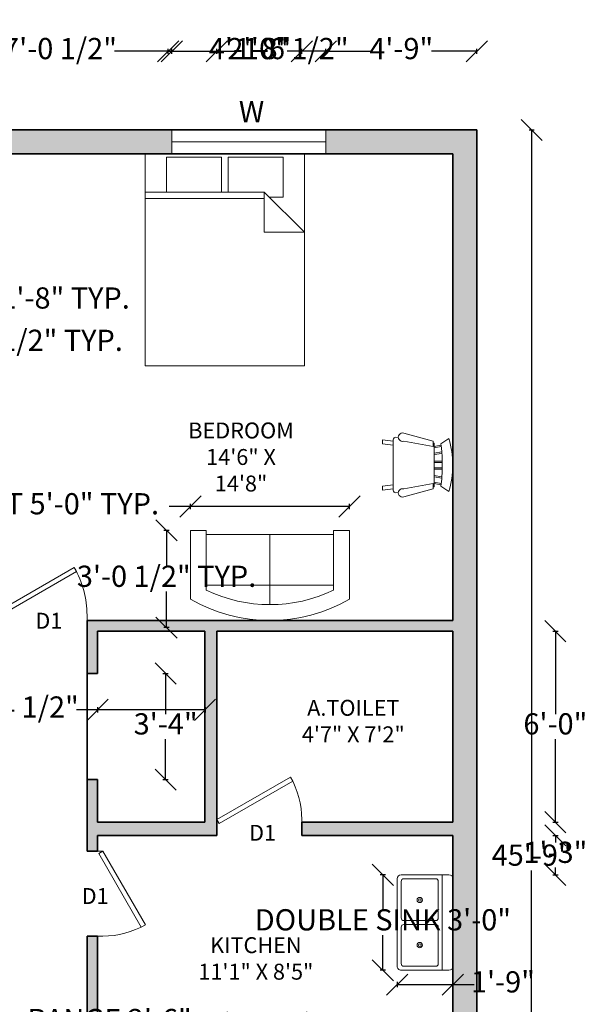
# Model space of a CAD drawing. Units: inches. Extents: x 2530 to 3100, y 543 to 1175.
# Tile 5 of 5: x 2883 to 3097, y 804 to 1175. Entities that reach past the tile are written whole.
import ezdxf

# ---------------------------------------------------------------- set-up
doc = ezdxf.new("R2010")
doc.units = ezdxf.units.IN
for name, color, linetype, lineweight in [('A-ANNO-DIMS', 2, 'Continuous', 18), ('A-ANNO-TEXT', 7, 'Continuous', 18), ('A-AREA-IDEN', 7, 'Continuous', 18), ('A-DOOR', 3, 'Continuous', 18), ('A-FLOR-FIXT', 8, 'Continuous', 18), ('A-FURN', 8, 'Continuous', 18), ('A-GLAZ', 4, 'Continuous', 18), ('A-WALL', 7, 'Continuous', 35), ('A-WALL-PATT', 30, 'Continuous', 13)]:
    doc.layers.add(name, color=color, linetype=linetype, lineweight=lineweight)
doc.styles.get("Standard").update_dxf_attribs({"font": 'arial.ttf'})
doc.dimstyles.new('ISO-25', dxfattribs={"dimtxt": 8, "dimasz": 8, "dimexe": 1, "dimexo": 1, "dimtad": 0, "dimtih": 1, "dimtoh": 1, "dimlunit": 3, "dimtxsty": 'Standard', "dimblk": 'OBLIQUE', "dimcen": 2.5, "dimadec": 0, "dimazin": 0, "dimtfac": 1, "dimtmove": 0, "dimatfit": 3, "dimfxl": 1, "dimfxlon": 1, "dimarcsym": 0})

# ---------------------------------------------------------------- blocks, each defined once
blk = doc.blocks.new('*U7')
for p, q in [((0, 0), (0, -6)), ((32, 0), (32, -6))]:
    blk.add_line(p, q)
blk.add_lwpolyline([(0, 0), (27.71, 16), (28.59, 14.48), (0.87, -1.52)], close=True)
blk.add_arc((0, 0), 32, 0, 30)
blk = doc.blocks.new('*U4')
for p, q in [((0, 0), (0, -6)), ((36, 0), (36, -6))]:
    blk.add_line(p, q)
blk.add_lwpolyline([(0, 0), (31.18, 18), (32.05, 16.48), (0.87, -1.52)], close=True)
blk.add_arc((0, 0), 36, 0, 30)
blk = doc.blocks.new('_Oblique')
at = {"color": 0, "linetype": 'ByBlock', "lineweight": -2}
blk.add_line((-0.5, -0.5), (0.5, 0.5), dxfattribs=at)
blk = doc.blocks.new('*D12')
at = {"layer": 'A-ANNO-DIMS', "color": 0, "lineweight": -2, "transparency": 16777216}
for p, q in [((3074.63, 1133.41), (3076.63, 1133.41)), ((3075.63, 1133.41), (3075.63, 863.62)), ((3075.63, 584.41), (3075.63, 854.2)), ((3074.63, 584.41), (3076.63, 584.41))]:
    blk.add_line(p, q, dxfattribs=at)
at = {"layer": 'Defpoints', "color": 0, "transparency": 16777216}
for p in [(3054.92, 1133.41), (3054.92, 584.41), (3075.63, 584.41)]:
    blk.add_point(p, dxfattribs=at)
at = {"layer": 'A-ANNO-DIMS', "color": 0, "lineweight": -2, "transparency": 16777216, "xscale": 8, "yscale": 8, "zscale": 8}
for p, rotation in [((3075.63, 1133.41), 90), ((3075.63, 584.41), 270)]:
    blk.add_blockref('_Oblique', p, dxfattribs=dict(at, rotation=rotation))
at = {"layer": 'A-ANNO-DIMS', "color": 0, "transparency": 16777216, "insert": (3075.63, 858.91), "char_height": 8, "attachment_point": 5}
blk.add_mtext('45\'-9"', dxfattribs=at)
blk = doc.blocks.new('Sink-double - 36 in top')
for p, q in [((-18, -4), (18, -4)), ((-0.75, -18.5), (-0.75, -6.5)), ((0.75, -6.5), (0.75, -18.5))]:
    blk.add_line(p, q)
for points in [[(-16.5, 0), (16.5, 0)], [(-18, -19.5), (-18, -1.5)], [(18, -1.5), (18, -19.5)], [(-16.5, -18.5), (-16.5, -6.5)], [(-15.5, -5.5), (-1.75, -5.5)], [(1.75, -5.5), (15.5, -5.5)], [(16.5, -6.5), (16.5, -18.5)], [(16.5, -21), (-16.5, -21)], [(-1.75, -19.5), (-15.5, -19.5)], [(15.5, -19.5), (1.75, -19.5)]]:
    blk.add_lwpolyline(points)
for centre, radius in [((-8.5, -12.5), 1), ((-8.5, -12.5), 0.5), ((8.5, -12.5), 1), ((8.5, -12.5), 0.5)]:
    blk.add_circle(centre, radius)
for centre, radius, start, end in [((-16.5, -1.5), 1.5, 90, 180), ((16.5, -1.5), 1.5, 0, 90), ((-15.5, -6.5), 1, 90, 180), ((-1.75, -6.5), 1, 0, 90), ((1.75, -6.5), 1, 90, 180), ((15.5, -6.5), 1, 0, 90), ((-15.5, -18.5), 1, 180, 270), ((-1.75, -18.5), 1, 270, 0), ((1.75, -18.5), 1, 180, 270), ((15.5, -18.5), 1, 270, 0), ((-16.5, -19.5), 1.5, 180, 270), ((16.5, -19.5), 1.5, 270, 0)]:
    blk.add_arc(centre, radius, start, end)
blk = doc.blocks.new('Bed - Queen')
for p, q in [((0, -80.00003), (0, 0)), ((0, 0), (59.99999, 0)), ((59.99999, 0), (59.99999, -80.00003)), ((7.99999, -1.2), (28.79998, -1.2)), ((7.99999, -14.4), (7.99999, -1.2)), ((28.79998, -1.2), (28.79998, -14.4)), ((31.19999, -1.2), (51.99999, -1.2)), ((31.19999, -14.4), (31.19999, -1.2)), ((51.99999, -1.2), (51.99999, -16.4)), ((0, -14.4), (44.8, -14.4)), ((59.99999, -29.6), (44.8, -14.4)), ((44.8, -14.4), (44.8, -29.6)), ((44.8, -16.8), (0, -16.8)), ((51.99999, -16.4), (46.79936, -16.4)), ((44.8, -29.6), (59.99999, -29.6)), ((59.99999, -80.00003), (0, -80.00003))]:
    blk.add_line(p, q)
blk = doc.blocks.new('Sofa - Roundback Loveseat 5 ft.')
for p, q in [((0, -32.44198), (0, -5.99998)), ((-24, -33.99998), (-24, -11.46958)), ((-23.9998, -13.38178), (23.99986, -13.38178)), ((24.00004, -33.99998), (24.00004, -11.46958)), ((-24, -32.44198), (24.00004, -32.44198))]:
    blk.add_line(p, q)
for points in [[(-24, -33.99998), (-30, -33.99998), (-30, -7.99998)], [(30.00004, -7.99998), (30.00004, -33.99998), (24.00004, -33.99998)]]:
    blk.add_lwpolyline(points)
for centre, radius, start, end in [((0, -60.24998), 60.24998, 60.13715, 119.8628), ((0, -61.38438), 55.38444, 64.32083, 115.6792)]:
    blk.add_arc(centre, radius, start, end)
blk = doc.blocks.new('Chair - Rocking')
for p, q in [((-8, -4.5), (-10, -1.5)), ((8, -4.5), (10, -1.5)), ((-8.23428, -6.99939), (-8.3093, -7.47958)), ((-8.23041, -7), (8.23915, -7)), ((-7.5, -4.5), (-7, -7)), ((-6.5, -7), (-7.02225, -4.43)), ((-4.5, -7), (-4.96674, -4.19951)), ((-4, -7), (-4.40532, -4.16272)), ((-1.5, -4.05012), (-1.5, -7)), ((-1, -7), (-1, -4.05012)), ((1, -7), (1, -4.04655)), ((1.5, -4.05012), (1.5, -7)), ((4, -7), (4.40187, -4.18694)), ((4.5, -7), (4.96761, -4.19437)), ((6.5, -7), (7, -4.4057)), ((7.5, -4.5), (7, -7)), ((8.31071, -7.48854), (8.23449, -7.00073)), ((-9, -7.5), (-12, -18.49999)), ((-7, -7.5), (-9, -7.5)), ((-9, -18.49999), (-7, -7.5)), ((7, -7.5), (9, -7.5)), ((9, -18.49999), (7, -7.5)), ((9, -7.5), (12, -18.49999)), ((-10.36644, -20.64523), (-10.5, -21.49999)), ((10.5, -21.49999), (10.3575, -20.58798)), ((-9, -22.49999), (-9.5, -26.49999)), ((0, -22.49999), (-9.5, -22.49999)), ((-8, -26.49999), (-7.5, -22.49999)), ((0, -22.49999), (9.5, -22.49999)), ((8, -26.49999), (7.5, -22.49999)), ((9, -22.49999), (9.5, -26.49999)), ((-9.5, -26.49999), (-8, -26.49999)), ((9.5, -26.49999), (8, -26.49999))]:
    blk.add_line(p, q)
for centre, radius, start, end in [((0, -34.08333), 34.08333, 72.93847, 107.0615), ((0, -68.25004), 64.25, 93.92211, 97.15267), ((0, -68.25004), 64.25, 82.84733, 93.92211), ((-10.5, -18.99999), 1.58114, 161.5651, 18.43495), ((10.5, -18.99999), 1.58114, 161.5651, 18.43495), ((-9.5, -21.49999), 1, 180, 270), ((9.5, -21.49999), 1, 270, 0)]:
    blk.add_arc(centre, radius, start, end)
blk = doc.blocks.new('*D24')
at = {"layer": 'A-ANNO-DIMS', "color": 0, "lineweight": -2, "transparency": 16777216}
for p, q in [((2946.92, 991.41), (2938.92, 991.41)), ((2946.92, 990.41), (2946.92, 992.41)), ((3006.92, 991.41), (2946.92, 991.41)), ((3006.92, 990.41), (3006.92, 992.41))]:
    blk.add_line(p, q, dxfattribs=at)
at = {"layer": 'Defpoints', "color": 0, "transparency": 16777216}
for p in [(2946.92, 991.41), (2946.92, 982.41), (3006.92, 982.41)]:
    blk.add_point(p, dxfattribs=at)
at = {"layer": 'A-ANNO-DIMS', "color": 0, "lineweight": -2, "transparency": 16777216, "xscale": 8, "yscale": 8, "zscale": 8, "rotation": 180}
blk.add_blockref('_Oblique', (2946.92, 991.41), dxfattribs=at)
at = {"layer": 'A-ANNO-DIMS', "color": 0, "lineweight": -2, "transparency": 16777216, "xscale": 8, "yscale": 8, "zscale": 8}
blk.add_blockref('_Oblique', (3006.92, 991.41), dxfattribs=at)
at = {"layer": 'A-ANNO-DIMS', "color": 0, "transparency": 16777216, "insert": (2883.03, 991.41), "char_height": 8, "attachment_point": 5}
blk.add_mtext('LOVESEAT 5\'-0" TYP.', dxfattribs=at)
blk = doc.blocks.new('*D25')
at = {"layer": 'A-ANNO-DIMS', "color": 0, "lineweight": -2, "transparency": 16777216}
for p, q in [((2938.92, 982.41), (2936.92, 982.41)), ((2937.92, 982.41), (2937.92, 968.84)), ((2937.92, 945.74), (2937.92, 959.31)), ((2938.92, 945.74), (2936.92, 945.74))]:
    blk.add_line(p, q, dxfattribs=at)
at = {"layer": 'Defpoints', "color": 0, "transparency": 16777216}
for p in [(2946.92, 982.41), (2937.92, 945.74), (2946.92, 945.74)]:
    blk.add_point(p, dxfattribs=at)
at = {"layer": 'A-ANNO-DIMS', "color": 0, "lineweight": -2, "transparency": 16777216, "xscale": 8, "yscale": 8, "zscale": 8}
for p, rotation in [((2937.92, 982.41), 90), ((2937.92, 945.74), 270)]:
    blk.add_blockref('_Oblique', p, dxfattribs=dict(at, rotation=rotation))
at = {"layer": 'A-ANNO-DIMS', "color": 0, "transparency": 16777216, "insert": (2937.92, 964.07), "char_height": 8, "attachment_point": 5}
blk.add_mtext('3\'-0 1/2" TYP.', dxfattribs=at)
blk = doc.blocks.new('*D30')
at = {"layer": 'A-ANNO-DIMS', "color": 0, "lineweight": -2, "transparency": 16777216}
for p, q in [((2869.69, 1065.33), (2871.69, 1065.33)), ((2870.69, 1065.33), (2870.69, 1057.81)), ((2870.69, 1040.78), (2870.69, 1048.29)), ((2869.69, 1040.78), (2871.69, 1040.78))]:
    blk.add_line(p, q, dxfattribs=at)
at = {"layer": 'Defpoints', "color": 0, "transparency": 16777216}
for p in [(2867.01, 1065.33), (2867.01, 1040.78), (2870.69, 1040.78)]:
    blk.add_point(p, dxfattribs=at)
at = {"layer": 'A-ANNO-DIMS', "color": 0, "lineweight": -2, "transparency": 16777216, "xscale": 8, "yscale": 8, "zscale": 8}
for p, rotation in [((2870.69, 1065.33), 90), ((2870.69, 1040.78), 270)]:
    blk.add_blockref('_Oblique', p, dxfattribs=dict(at, rotation=rotation))
at = {"layer": 'A-ANNO-DIMS', "color": 0, "transparency": 16777216, "insert": (2870.69, 1053.05), "char_height": 8, "attachment_point": 5}
blk.add_mtext('BASIN 2\'-0 1/2" TYP.', dxfattribs=at)
blk = doc.blocks.new('*D31')
at = {"layer": 'A-ANNO-DIMS', "color": 0, "lineweight": -2, "transparency": 16777216}
for p, q in [((2846.87, 1068.01), (2846.87, 1070.01)), ((2867.01, 1068.01), (2867.01, 1070.01)), ((2846.87, 1069.01), (2867.01, 1069.01)), ((2867.01, 1069.01), (2875.01, 1069.01))]:
    blk.add_line(p, q, dxfattribs=at)
at = {"layer": 'Defpoints', "color": 0, "transparency": 16777216}
for p in [(2867.01, 1069.01), (2846.87, 1065.33), (2867.01, 1065.33)]:
    blk.add_point(p, dxfattribs=at)
at = {"layer": 'A-ANNO-DIMS', "color": 0, "lineweight": -2, "transparency": 16777216, "xscale": 8, "yscale": 8, "zscale": 8, "rotation": 180}
blk.add_blockref('_Oblique', (2846.87, 1069.01), dxfattribs=at)
at = {"layer": 'A-ANNO-DIMS', "color": 0, "lineweight": -2, "transparency": 16777216, "xscale": 8, "yscale": 8, "zscale": 8}
blk.add_blockref('_Oblique', (2867.01, 1069.01), dxfattribs=at)
at = {"layer": 'A-ANNO-DIMS', "color": 0, "transparency": 16777216, "insert": (2899.64, 1069.01), "char_height": 8, "attachment_point": 5}
blk.add_mtext('1\'-8" TYP.', dxfattribs=at)
blk = doc.blocks.new('*D34')
at = {"layer": 'A-ANNO-DIMS', "color": 0, "lineweight": -2, "transparency": 16777216}
for p, q in [((3020.52, 852.52), (3018.52, 852.52)), ((3019.52, 852.52), (3019.52, 839.29)), ((3019.52, 816.52), (3019.52, 829.76)), ((3020.52, 816.52), (3018.52, 816.52))]:
    blk.add_line(p, q, dxfattribs=at)
at = {"layer": 'Defpoints', "color": 0, "transparency": 16777216}
for p in [(3024.92, 852.52), (3019.52, 816.52), (3024.92, 816.52)]:
    blk.add_point(p, dxfattribs=at)
at = {"layer": 'A-ANNO-DIMS', "color": 0, "lineweight": -2, "transparency": 16777216, "xscale": 8, "yscale": 8, "zscale": 8}
for p, rotation in [((3019.52, 852.52), 90), ((3019.52, 816.52), 270)]:
    blk.add_blockref('_Oblique', p, dxfattribs=dict(at, rotation=rotation))
at = {"layer": 'A-ANNO-DIMS', "color": 0, "transparency": 16777216, "insert": (3019.52, 834.52), "char_height": 8, "attachment_point": 5}
blk.add_mtext('DOUBLE SINK 3\'-0"', dxfattribs=at)
blk = doc.blocks.new('*D35')
at = {"layer": 'A-ANNO-DIMS', "color": 0, "lineweight": -2, "transparency": 16777216}
for p, q in [((3024.92, 812.12), (3024.92, 810.12)), ((3024.92, 811.12), (3045.92, 811.12)), ((3045.92, 812.12), (3045.92, 810.12)), ((3045.92, 811.12), (3053.92, 811.12))]:
    blk.add_line(p, q, dxfattribs=at)
at = {"layer": 'Defpoints', "color": 0, "transparency": 16777216}
for p in [(3024.92, 816.52), (3045.92, 816.52), (3045.92, 811.12)]:
    blk.add_point(p, dxfattribs=at)
at = {"layer": 'A-ANNO-DIMS', "color": 0, "lineweight": -2, "transparency": 16777216, "xscale": 8, "yscale": 8, "zscale": 8, "rotation": 180}
blk.add_blockref('_Oblique', (3024.92, 811.12), dxfattribs=at)
at = {"layer": 'A-ANNO-DIMS', "color": 0, "lineweight": -2, "transparency": 16777216, "xscale": 8, "yscale": 8, "zscale": 8}
blk.add_blockref('_Oblique', (3045.92, 811.12), dxfattribs=at)
at = {"layer": 'A-ANNO-DIMS', "color": 0, "transparency": 16777216, "insert": (3064.8, 811.12), "char_height": 8, "attachment_point": 5}
blk.add_mtext('1\'-9"', dxfattribs=at)
blk = doc.blocks.new('*D36')
at = {"layer": 'A-ANNO-DIMS', "color": 0, "lineweight": -2, "transparency": 16777216}
for p, q in [((2956.92, 796.91), (2948.92, 796.91)), ((2956.92, 795.91), (2956.92, 797.91)), ((2986.92, 796.91), (2956.92, 796.91)), ((2986.92, 795.91), (2986.92, 797.91))]:
    blk.add_line(p, q, dxfattribs=at)
at = {"layer": 'Defpoints', "color": 0, "transparency": 16777216}
for p in [(2956.92, 796.91), (2956.92, 792.41), (2986.92, 792.41)]:
    blk.add_point(p, dxfattribs=at)
at = {"layer": 'A-ANNO-DIMS', "color": 0, "lineweight": -2, "transparency": 16777216, "xscale": 8, "yscale": 8, "zscale": 8, "rotation": 180}
blk.add_blockref('_Oblique', (2956.92, 796.91), dxfattribs=at)
at = {"layer": 'A-ANNO-DIMS', "color": 0, "lineweight": -2, "transparency": 16777216, "xscale": 8, "yscale": 8, "zscale": 8}
blk.add_blockref('_Oblique', (2986.92, 796.91), dxfattribs=at)
at = {"layer": 'A-ANNO-DIMS', "color": 0, "transparency": 16777216, "insert": (2916.44, 796.91), "char_height": 8, "attachment_point": 5}
blk.add_mtext('RANGE 2\'-6"', dxfattribs=at)
blk = doc.blocks.new('*D38')
at = {"layer": 'A-ANNO-DIMS', "color": 0, "lineweight": -2, "transparency": 16777216}
for p, q in [((2911.92, 791.86), (2903.92, 791.86)), ((2911.92, 790.86), (2911.92, 792.86)), ((2938.56, 791.86), (2911.92, 791.86)), ((2938.56, 790.86), (2938.56, 792.86))]:
    blk.add_line(p, q, dxfattribs=at)
at = {"layer": 'Defpoints', "color": 0, "transparency": 16777216}
for p in [(2911.92, 791.86), (2911.92, 787.87), (2938.56, 787.87)]:
    blk.add_point(p, dxfattribs=at)
at = {"layer": 'A-ANNO-DIMS', "color": 0, "lineweight": -2, "transparency": 16777216, "xscale": 8, "yscale": 8, "zscale": 8, "rotation": 180}
blk.add_blockref('_Oblique', (2911.92, 791.86), dxfattribs=at)
at = {"layer": 'A-ANNO-DIMS', "color": 0, "lineweight": -2, "transparency": 16777216, "xscale": 8, "yscale": 8, "zscale": 8}
blk.add_blockref('_Oblique', (2938.56, 791.86), dxfattribs=at)
at = {"layer": 'A-ANNO-DIMS', "color": 0, "transparency": 16777216, "insert": (2837.6, 791.86), "char_height": 8, "attachment_point": 5}
blk.add_mtext('REFRIGERATOR 2\'-2 1/2"', dxfattribs=at)
blk = doc.blocks.new('*D54')
at = {"layer": 'A-ANNO-DIMS', "color": 0, "lineweight": -2, "transparency": 16777216}
for p, q in [((2855.56, 1162.06), (2855.56, 1164.06)), ((2855.56, 1163.06), (2877.19, 1163.06)), ((2939.91, 1163.06), (2918.28, 1163.06)), ((2939.91, 1162.06), (2939.91, 1164.06))]:
    blk.add_line(p, q, dxfattribs=at)
at = {"layer": 'Defpoints', "color": 0, "transparency": 16777216}
for p in [(2939.91, 1163.06), (2855.56, 1133.41), (2939.91, 1133.41)]:
    blk.add_point(p, dxfattribs=at)
at = {"layer": 'A-ANNO-DIMS', "color": 0, "lineweight": -2, "transparency": 16777216, "xscale": 8, "yscale": 8, "zscale": 8, "rotation": 180}
blk.add_blockref('_Oblique', (2855.56, 1163.06), dxfattribs=at)
at = {"layer": 'A-ANNO-DIMS', "color": 0, "lineweight": -2, "transparency": 16777216, "xscale": 8, "yscale": 8, "zscale": 8}
blk.add_blockref('_Oblique', (2939.91, 1163.06), dxfattribs=at)
at = {"layer": 'A-ANNO-DIMS', "color": 0, "transparency": 16777216, "insert": (2897.74, 1163.06), "char_height": 8, "attachment_point": 5}
blk.add_mtext('7\'-0 1/2"', dxfattribs=at)
blk = doc.blocks.new('*D55')
at = {"layer": 'A-ANNO-DIMS', "color": 0, "lineweight": -2, "transparency": 16777216}
for p, q in [((2939.91, 1162.06), (2939.91, 1164.06)), ((2939.91, 1163.06), (2954.41, 1163.06)), ((2997.97, 1163.06), (2983.47, 1163.06)), ((2997.97, 1162.06), (2997.97, 1164.06))]:
    blk.add_line(p, q, dxfattribs=at)
at = {"layer": 'Defpoints', "color": 0, "transparency": 16777216}
for p in [(2997.97, 1163.06), (2939.91, 1133.41), (2997.97, 1133.41)]:
    blk.add_point(p, dxfattribs=at)
at = {"layer": 'A-ANNO-DIMS', "color": 0, "lineweight": -2, "transparency": 16777216, "xscale": 8, "yscale": 8, "zscale": 8, "rotation": 180}
blk.add_blockref('_Oblique', (2939.91, 1163.06), dxfattribs=at)
at = {"layer": 'A-ANNO-DIMS', "color": 0, "lineweight": -2, "transparency": 16777216, "xscale": 8, "yscale": 8, "zscale": 8}
blk.add_blockref('_Oblique', (2997.97, 1163.06), dxfattribs=at)
at = {"layer": 'A-ANNO-DIMS', "color": 0, "transparency": 16777216, "insert": (2968.94, 1163.06), "char_height": 8, "attachment_point": 5}
blk.add_mtext('4\'-10"', dxfattribs=at)
blk = doc.blocks.new('*D65')
at = {"layer": 'A-ANNO-DIMS', "color": 0, "lineweight": -2, "transparency": 16777216}
for p, q in [((2597.27, 861.41), (2595.27, 861.41)), ((2596.27, 861.41), (2596.27, 850.12)), ((2596.27, 829.41), (2596.27, 840.7)), ((2597.27, 829.41), (2595.27, 829.41))]:
    blk.add_line(p, q, dxfattribs=at)
at = {"layer": 'Defpoints', "color": 0, "transparency": 16777216}
for p in [(2596.27, 861.41), (2907.92, 861.41), (2907.92, 829.41)]:
    blk.add_point(p, dxfattribs=at)
at = {"layer": 'A-ANNO-DIMS', "color": 0, "lineweight": -2, "transparency": 16777216, "xscale": 8, "yscale": 8, "zscale": 8}
for p, rotation in [((2596.27, 861.41), 90), ((2596.27, 829.41), 270)]:
    blk.add_blockref('_Oblique', p, dxfattribs=dict(at, rotation=rotation))
at = {"layer": 'A-ANNO-DIMS', "color": 0, "transparency": 16777216, "insert": (2596.27, 845.41), "char_height": 8, "attachment_point": 5}
blk.add_mtext('2\'-8"', dxfattribs=at)
blk = doc.blocks.new('*D69')
at = {"layer": 'A-ANNO-DIMS', "color": 0, "lineweight": -2, "transparency": 16777216}
for p, q in [((2956.92, 555.76), (2956.92, 553.76)), ((2956.92, 554.76), (2990.19, 554.76)), ((3045.92, 554.76), (3012.64, 554.76)), ((3045.92, 555.76), (3045.92, 553.76))]:
    blk.add_line(p, q, dxfattribs=at)
at = {"layer": 'Defpoints', "color": 0, "transparency": 16777216}
for p in [(2956.92, 944.41), (3045.92, 944.41), (3045.92, 554.76)]:
    blk.add_point(p, dxfattribs=at)
at = {"layer": 'A-ANNO-DIMS', "color": 0, "lineweight": -2, "transparency": 16777216, "xscale": 8, "yscale": 8, "zscale": 8, "rotation": 180}
blk.add_blockref('_Oblique', (2956.92, 554.76), dxfattribs=at)
at = {"layer": 'A-ANNO-DIMS', "color": 0, "lineweight": -2, "transparency": 16777216, "xscale": 8, "yscale": 8, "zscale": 8}
blk.add_blockref('_Oblique', (3045.92, 554.76), dxfattribs=at)
at = {"layer": 'A-ANNO-DIMS', "color": 0, "transparency": 16777216, "insert": (3001.42, 554.76), "char_height": 8, "attachment_point": 5}
blk.add_mtext('7\'-5"', dxfattribs=at)
blk = doc.blocks.new('*D70')
at = {"layer": 'A-ANNO-DIMS', "color": 0, "lineweight": -2, "transparency": 16777216}
for p, q in [((3083.57, 944.41), (3085.57, 944.41)), ((3084.57, 944.41), (3084.57, 913.12)), ((3084.57, 872.41), (3084.57, 903.7)), ((3083.57, 872.41), (3085.57, 872.41))]:
    blk.add_line(p, q, dxfattribs=at)
at = {"layer": 'Defpoints', "color": 0, "transparency": 16777216}
for p in [(3045.92, 944.41), (3084.57, 944.41), (3045.92, 872.41)]:
    blk.add_point(p, dxfattribs=at)
at = {"layer": 'A-ANNO-DIMS', "color": 0, "lineweight": -2, "transparency": 16777216, "xscale": 8, "yscale": 8, "zscale": 8}
for p, rotation in [((3084.57, 944.41), 90), ((3084.57, 872.41), 270)]:
    blk.add_blockref('_Oblique', p, dxfattribs=dict(at, rotation=rotation))
at = {"layer": 'A-ANNO-DIMS', "color": 0, "transparency": 16777216, "insert": (3084.57, 908.41), "char_height": 8, "attachment_point": 5}
blk.add_mtext('6\'-0"', dxfattribs=at)
blk = doc.blocks.new('*D73')
at = {"layer": 'A-ANNO-DIMS', "color": 0, "lineweight": -2, "transparency": 16777216}
for p, q in [((2997.97, 1162.06), (2997.97, 1164.06)), ((2997.97, 1163.06), (3015.02, 1163.06)), ((3054.92, 1163.06), (3037.86, 1163.06)), ((3054.92, 1162.06), (3054.92, 1164.06))]:
    blk.add_line(p, q, dxfattribs=at)
at = {"layer": 'Defpoints', "color": 0, "transparency": 16777216}
for p in [(3054.92, 1163.06), (2997.97, 1133.41), (3054.92, 1133.41)]:
    blk.add_point(p, dxfattribs=at)
at = {"layer": 'A-ANNO-DIMS', "color": 0, "lineweight": -2, "transparency": 16777216, "xscale": 8, "yscale": 8, "zscale": 8, "rotation": 180}
blk.add_blockref('_Oblique', (2997.97, 1163.06), dxfattribs=at)
at = {"layer": 'A-ANNO-DIMS', "color": 0, "lineweight": -2, "transparency": 16777216, "xscale": 8, "yscale": 8, "zscale": 8}
blk.add_blockref('_Oblique', (3054.92, 1163.06), dxfattribs=at)
at = {"layer": 'A-ANNO-DIMS', "color": 0, "transparency": 16777216, "insert": (3026.44, 1163.06), "char_height": 8, "attachment_point": 5}
blk.add_mtext('4\'-9"', dxfattribs=at)
blk = doc.blocks.new('*D75')
at = {"layer": 'A-ANNO-DIMS', "color": 0, "lineweight": -2, "transparency": 16777216}
for p, q in [((2936.57, 928.41), (2938.57, 928.41)), ((2937.57, 928.41), (2937.57, 913.12)), ((2937.57, 888.41), (2937.57, 903.7)), ((2936.57, 888.41), (2938.57, 888.41))]:
    blk.add_line(p, q, dxfattribs=at)
at = {"layer": 'Defpoints', "color": 0, "transparency": 16777216}
for p in [(2907.92, 928.41), (2907.92, 888.41), (2937.57, 888.41)]:
    blk.add_point(p, dxfattribs=at)
at = {"layer": 'A-ANNO-DIMS', "color": 0, "lineweight": -2, "transparency": 16777216, "xscale": 8, "yscale": 8, "zscale": 8}
for p, rotation in [((2937.57, 928.41), 90), ((2937.57, 888.41), 270)]:
    blk.add_blockref('_Oblique', p, dxfattribs=dict(at, rotation=rotation))
at = {"layer": 'A-ANNO-DIMS', "color": 0, "transparency": 16777216, "insert": (2937.57, 908.41), "char_height": 8, "attachment_point": 5}
blk.add_mtext('3\'-4"', dxfattribs=at)
blk = doc.blocks.new('*D76')
at = {"layer": 'A-ANNO-DIMS', "color": 0, "lineweight": -2, "transparency": 16777216}
for p, q in [((2911.92, 914.76), (2903.92, 914.76)), ((2911.92, 915.76), (2911.92, 913.76)), ((2952.42, 914.76), (2911.92, 914.76)), ((2952.42, 915.76), (2952.42, 913.76))]:
    blk.add_line(p, q, dxfattribs=at)
at = {"layer": 'Defpoints', "color": 0, "transparency": 16777216}
for p in [(2911.92, 944.41), (2952.42, 944.41), (2911.92, 914.76)]:
    blk.add_point(p, dxfattribs=at)
at = {"layer": 'A-ANNO-DIMS', "color": 0, "lineweight": -2, "transparency": 16777216, "xscale": 8, "yscale": 8, "zscale": 8}
for p, rotation in [((2911.92, 914.76), 180.000000000001), ((2952.42, 914.76), 1.0392e-12)]:
    blk.add_blockref('_Oblique', p, dxfattribs=dict(at, rotation=rotation))
at = {"layer": 'A-ANNO-DIMS', "color": 0, "transparency": 16777216, "insert": (2883.34, 914.76), "char_height": 8, "attachment_point": 5}
blk.add_mtext('3\'-4 1/2"', dxfattribs=at)
blk = doc.blocks.new('*D77')
at = {"layer": 'A-ANNO-DIMS', "color": 0, "lineweight": -2, "transparency": 16777216}
for p, q in [((2938.56, 1162.06), (2938.56, 1164.06)), ((2938.56, 1163.06), (2956.92, 1163.06)), ((2956.92, 1162.06), (2956.92, 1164.06)), ((2956.92, 1163.06), (2964.92, 1163.06))]:
    blk.add_line(p, q, dxfattribs=at)
at = {"layer": 'Defpoints', "color": 0, "transparency": 16777216}
for p in [(2956.92, 1163.06), (2956.92, 790.41), (2938.56, 787.13)]:
    blk.add_point(p, dxfattribs=at)
at = {"layer": 'A-ANNO-DIMS', "color": 0, "lineweight": -2, "transparency": 16777216, "xscale": 8, "yscale": 8, "zscale": 8, "rotation": 180}
blk.add_blockref('_Oblique', (2938.56, 1163.06), dxfattribs=at)
at = {"layer": 'A-ANNO-DIMS', "color": 0, "lineweight": -2, "transparency": 16777216, "xscale": 8, "yscale": 8, "zscale": 8}
blk.add_blockref('_Oblique', (2956.92, 1163.06), dxfattribs=at)
at = {"layer": 'A-ANNO-DIMS', "color": 0, "transparency": 16777216, "insert": (2985.12, 1163.06), "char_height": 8, "attachment_point": 5}
blk.add_mtext('1\'-6 1/2"', dxfattribs=at)
blk = doc.blocks.new('*D78')
at = {"layer": 'A-ANNO-DIMS', "color": 0, "lineweight": -2, "transparency": 16777216}
for p, q in [((3083.57, 867.41), (3085.57, 867.41)), ((3084.57, 867.41), (3084.57, 864.68)), ((3084.57, 852.52), (3084.57, 855.25)), ((3083.57, 852.52), (3085.57, 852.52))]:
    blk.add_line(p, q, dxfattribs=at)
at = {"layer": 'Defpoints', "color": 0, "transparency": 16777216}
for p in [(3045.92, 867.41), (3084.57, 867.41), (3044.42, 852.52)]:
    blk.add_point(p, dxfattribs=at)
at = {"layer": 'A-ANNO-DIMS', "color": 0, "lineweight": -2, "transparency": 16777216, "xscale": 8, "yscale": 8, "zscale": 8}
for p, rotation in [((3084.57, 867.41), 90), ((3084.57, 852.52), 270)]:
    blk.add_blockref('_Oblique', p, dxfattribs=dict(at, rotation=rotation))
at = {"layer": 'A-ANNO-DIMS', "color": 0, "transparency": 16777216, "insert": (3084.57, 859.97), "char_height": 8, "attachment_point": 5}
blk.add_mtext('1\'-3"', dxfattribs=at)
blk = doc.blocks.new('*D82')
at = {"layer": 'A-ANNO-DIMS', "color": 0, "lineweight": -2, "transparency": 16777216}
for p, q in [((2956.92, 1162.06), (2956.92, 1164.06)), ((2956.92, 1163.06), (2961.59, 1163.06)), ((2988.92, 1163.06), (2984.24, 1163.06)), ((2988.92, 1162.06), (2988.92, 1164.06))]:
    blk.add_line(p, q, dxfattribs=at)
at = {"layer": 'Defpoints', "color": 0, "transparency": 16777216}
for p in [(2988.92, 1163.06), (2956.92, 867.41), (2988.92, 867.41)]:
    blk.add_point(p, dxfattribs=at)
at = {"layer": 'A-ANNO-DIMS', "color": 0, "lineweight": -2, "transparency": 16777216, "xscale": 8, "yscale": 8, "zscale": 8, "rotation": 180}
blk.add_blockref('_Oblique', (2956.92, 1163.06), dxfattribs=at)
at = {"layer": 'A-ANNO-DIMS', "color": 0, "lineweight": -2, "transparency": 16777216, "xscale": 8, "yscale": 8, "zscale": 8}
blk.add_blockref('_Oblique', (2988.92, 1163.06), dxfattribs=at)
at = {"layer": 'A-ANNO-DIMS', "color": 0, "transparency": 16777216, "insert": (2972.92, 1163.06), "char_height": 8, "attachment_point": 5}
blk.add_mtext('2\'-8"', dxfattribs=at)

msp = doc.modelspace()

# ---------------------------------------------------------------- hatches: boundary and pattern name
at = {"layer": 'A-WALL-PATT'}
h = msp.add_hatch(color=256, dxfattribs=at)
h.dxf.hatch_style = 1
h.paths.add_polyline_path([(2676.945, 1133.407), (2625.918, 1133.407), (2625.918, 584.407), (2673.585, 584.407), (2673.585, 593.407), (2634.918, 593.407), (2634.918, 757.407), (2717.918, 757.407), (2717.918, 766.407), (2634.918, 766.407), (2634.918, 944.407), (2772.918, 944.407), (2772.918, 948.407), (2634.918, 948.407), (2634.918, 1124.407), (2676.945, 1124.407)])
h.paths.add_polyline_path([(2822.346, 1133.407), (2739.946, 1133.407), (2739.946, 1124.407), (2808.918, 1124.407), (2808.918, 1070.407), (2812.918, 1070.407), (2812.918, 1124.407), (2822.346, 1124.407)])
h.paths.add_polyline_path([(2939.91, 1133.407), (2855.561, 1133.407), (2855.561, 1124.407), (2867.918, 1124.407), (2867.918, 1038.407), (2808.918, 1038.407), (2808.918, 944.407), (2871.918, 944.407), (2871.918, 1002.407), (2867.918, 1002.407), (2867.918, 948.407), (2812.918, 948.407), (2812.918, 1034.407), (2871.918, 1034.407), (2871.918, 1124.407), (2939.91, 1124.407)])
h.paths.add_polyline_path([(3054.918, 1133.407), (2997.969, 1133.407), (2997.969, 1124.407), (3045.918, 1124.407), (3045.918, 948.407), (2907.918, 948.407), (2907.918, 928.407), (2911.918, 928.407), (2911.918, 944.407), (2952.418, 944.407), (2952.418, 872.407), (2911.918, 872.407), (2911.918, 888.407), (2907.918, 888.407), (2907.918, 861.407), (2911.918, 861.407), (2911.918, 867.407), (2956.918, 867.407), (2956.918, 944.407), (3045.918, 944.407), (3045.918, 872.407), (2988.918, 872.407), (2988.918, 867.407), (3045.918, 867.407), (3045.918, 766.407), (2986.918, 766.407), (2986.918, 757.407), (3045.918, 757.407), (3045.918, 593.407), (2906.263, 593.407), (2906.263, 584.407), (3054.918, 584.407)])
h.paths.add_polyline_path([(2780.418, 593.407), (2762.418, 593.407), (2762.418, 693.907), (2757.918, 693.907), (2757.918, 593.407), (2719.35, 593.407), (2719.35, 584.407), (2780.418, 584.407)])
h.paths.add_polyline_path([(2846.356, 593.407), (2826.918, 593.407), (2826.918, 757.407), (2826.918, 766.407), (2822.418, 766.407), (2822.418, 693.907), (2794.418, 693.907), (2794.418, 689.407), (2822.418, 689.407), (2822.418, 593.407), (2804.418, 593.407), (2804.418, 584.407), (2846.356, 584.407)])
h.paths.add_polyline_path([(2938.918, 766.407), (2911.918, 766.407), (2911.918, 829.407), (2907.918, 829.407), (2907.918, 766.407), (2886.918, 766.407), (2886.918, 757.407), (2938.918, 757.407)])
h.paths.add_polyline_path([(2822.418, 766.407), (2757.918, 766.407), (2757.918, 757.407), (2757.918, 721.407), (2762.418, 721.407), (2762.418, 757.407), (2822.418, 757.407)])

# ---------------------------------------------------------------- linework, layer by layer
at = {"layer": 'A-GLAZ'}
for p, q in [((2939.91, 1124.407), (2939.91, 1133.407)), ((2997.969, 1124.407), (2997.969, 1133.407)), ((2997.969, 1128.907), (2939.91, 1128.907))]:
    msp.add_line(p, q, dxfattribs=at)
at = {"layer": 'A-WALL'}
for p, q in [((3054.918, 1133.407), (2625.918, 1133.407)), ((3054.918, 584.407), (3054.918, 1133.407)), ((3045.918, 1124.407), (2871.918, 1124.407)), ((3045.918, 948.407), (3045.918, 1124.407)), ((3045.918, 948.407), (2907.918, 948.407)), ((2907.918, 861.407), (2907.918, 948.407)), ((2952.418, 944.407), (2911.918, 944.407)), ((2911.918, 928.407), (2911.918, 944.407)), ((2952.418, 872.407), (2952.418, 944.407)), ((3045.918, 944.407), (2956.918, 944.407)), ((2956.918, 867.407), (2956.918, 944.407)), ((3045.918, 872.407), (3045.918, 944.407)), ((2911.918, 928.407), (2907.918, 928.407)), ((2911.918, 888.407), (2907.918, 888.407)), ((2911.918, 872.407), (2911.918, 888.407)), ((2952.418, 872.407), (2911.918, 872.407)), ((3045.918, 872.407), (2988.918, 872.407)), ((2988.918, 867.407), (2988.918, 872.407)), ((2956.918, 867.407), (2911.918, 867.407)), ((2911.918, 861.407), (2911.918, 867.407)), ((3045.918, 867.407), (2988.918, 867.407)), ((3045.918, 766.407), (3045.918, 867.407)), ((2911.918, 861.407), (2907.918, 861.407)), ((2907.918, 766.407), (2907.918, 829.407)), ((2911.918, 829.407), (2907.918, 829.407)), ((2911.918, 766.407), (2911.918, 829.407))]:
    msp.add_line(p, q, dxfattribs=at)

# ---------------------------------------------------------------- block references
at = {"layer": 'A-DOOR'}
for name, p in [('*U4', (2871.918, 950.407)), ('*U7', (2956.918, 873.407))]:
    msp.add_blockref(name, p, dxfattribs=at)
at = {"layer": 'A-DOOR', "rotation": 270}
msp.add_blockref('*U7', (2913.918, 861.407), dxfattribs=at)
at = {"layer": 'A-FLOR-FIXT', "rotation": 270}
msp.add_blockref('Sink-double - 36 in top', (3045.918, 834.525), dxfattribs=at)
at = {"layer": 'A-FURN'}
msp.add_blockref('Bed - Queen', (2929.896, 1124.407), dxfattribs=at)
at = {"layer": 'A-FURN', "xscale": -1, "rotation": 270}
msp.add_blockref('Chair - Rocking', (3045.918, 1007.054), dxfattribs=at)
at = {"layer": 'A-FURN', "rotation": 180}
msp.add_blockref('Sofa - Roundback Loveseat 5 ft.', (2976.918, 948.407), dxfattribs=at)

# ---------------------------------------------------------------- texts
at = {"layer": 'A-ANNO-TEXT', "attachment_point": 1}
for s, insert, char_height in [('\\pxqc;W', (2960.729, 1144.337), 8), ('\\pxqc;D1', (2884.271, 951.328), 6), ('\\pxqc;D1', (2964.892, 871.371), 6), ('\\pxqc;D1', (2901.741, 847.52), 6)]:
    msp.add_mtext_dynamic_manual_height_columns(s, width=18.48176, gutter_width=12.5, heights=[0], dxfattribs=dict(at, insert=insert, char_height=char_height))
at = {"layer": 'A-AREA-IDEN', "char_height": 6, "attachment_point": 1}
for s, insert in [('\\pxqc;BEDROOM\\P14\'6" X 14\'8"', (2942.179, 1023.084)), ('\\pxqc;A.TOILET\\P4\'7" X 7\'2"', (2984.53, 918.5)), ('\\pxqc;KITCHEN\\P11\'1" X 8\'5"', (2947.776, 828.988))]:
    msp.add_mtext_dynamic_manual_height_columns(s, width=47.65744, gutter_width=12.5, heights=[0], dxfattribs=dict(at, insert=insert))

# ---------------------------------------------------------------- dimensions: what is measured, and where the dimension line sits
at = {"layer": 'A-ANNO-DIMS'}
for base, p1, p2, picture, middle in [((2939.91, 1163.057), (2855.561, 1133.407), (2939.91, 1133.407), '*D54', (2897.736, 1163.057)), ((2956.918, 1163.057), (2938.558, 787.128), (2956.918, 790.407), '*D77', (2985.12, 1163.057)), ((2997.969, 1163.057), (2939.91, 1133.407), (2997.969, 1133.407), '*D55', (2968.94, 1163.057)), ((2988.918, 1163.057), (2956.918, 867.407), (2988.918, 867.407), '*D82', (2972.918, 1163.057)), ((3054.918, 1163.057), (2997.969, 1133.407), (3054.918, 1133.407), '*D73', (3026.443, 1163.057)), ((3045.918, 554.757), (2956.918, 944.407), (3045.918, 944.407), '*D69', (3001.418, 554.757)), ((3045.918, 811.125), (3024.918, 816.525), (3045.918, 816.525), '*D35', (3064.799, 811.125))]:
    dim = msp.add_linear_dim(base=base, p1=p1, p2=p2, dimstyle='ISO-25', override={"dimdec": 1, "dimlfac": 1, "dimrnd": 0, "dimzin": 1, "dimdsep": 46, "dimlunit": 4, "dimfrac": 2}, dxfattribs=at)
    dim.commit()
    dim.dimension.update_dxf_attribs({"geometry": picture, "text_midpoint": middle})
for base, p1, p2, angle, override, picture, middle in [((3075.63, 584.407), (3054.918, 1133.407), (3054.918, 584.407), 90, {"dimclrd": 0, "dimclre": 0, "dimclrt": 0}, '*D12', (3075.63, 858.907)), ((3084.568, 944.407), (3045.918, 872.407), (3045.918, 944.407), 90, {"dimdec": 1, "dimlfac": 1, "dimrnd": 0, "dimzin": 1, "dimdsep": 46, "dimlunit": 4, "dimfrac": 2}, '*D70', (3084.568, 908.407)), ((2911.918, 914.757), (2952.418, 944.407), (2911.918, 944.407), 180, {"dimdec": 1, "dimlfac": 1, "dimrnd": 0, "dimzin": 1, "dimdsep": 46, "dimlunit": 4, "dimfrac": 2}, '*D76', (2883.342, 914.757)), ((2937.568, 888.407), (2907.918, 928.407), (2907.918, 888.407), 270, {"dimdec": 1, "dimlfac": 1, "dimrnd": 0, "dimzin": 1, "dimdsep": 46, "dimlunit": 4, "dimfrac": 2}, '*D75', (2937.568, 908.407)), ((3084.568, 867.407), (3044.418, 852.525), (3045.918, 867.407), 90, {"dimdec": 1, "dimlfac": 1, "dimrnd": 0, "dimzin": 1, "dimdsep": 46, "dimlunit": 4, "dimfrac": 2}, '*D78', (3084.568, 859.966)), ((2596.268, 861.407), (2907.918, 829.407), (2907.918, 861.407), 90, {"dimdec": 1, "dimlfac": 1, "dimrnd": 0, "dimzin": 1, "dimdsep": 46, "dimlunit": 4, "dimfrac": 2}, '*D65', (2596.268, 845.407))]:
    dim = msp.add_linear_dim(base=base, p1=p1, p2=p2, angle=angle, dimstyle='ISO-25', override=override, dxfattribs=at)
    dim.commit()
    dim.dimension.update_dxf_attribs({"geometry": picture, "text_midpoint": middle})
dim = msp.add_linear_dim(base=(2867.011, 1069.011), p1=(2846.874, 1065.328), p2=(2867.011, 1065.328), text='<> TYP.', dimstyle='ISO-25', override={"dimdec": 1, "dimlfac": 1, "dimrnd": 0, "dimzin": 1, "dimdsep": 46, "dimlunit": 4, "dimfrac": 2}, dxfattribs=at)
dim.commit()
dim.dimension.update_dxf_attribs({"geometry": '*D31', "text_midpoint": (2899.641, 1069.011)})
for base, p1, p2, angle, text, picture, middle in [((2870.6936, 1040.7776), (2867.011, 1065.3285), (2867.011, 1040.7776), 270, 'BASIN <> TYP.', '*D30', (2870.6936, 1053.053)), ((2946.917, 991.407), (3006.918, 982.407), (2946.917, 982.407), 180, 'LOVESEAT <> TYP.', '*D24', (2883.032, 991.407)), ((2937.917, 945.741), (2946.917, 982.407), (2946.917, 945.741), 270, '<> TYP.', '*D25', (2937.917, 964.074)), ((3019.518, 816.525), (3024.918, 852.525), (3024.918, 816.525), 270, 'DOUBLE SINK <>', '*D34', (3019.518, 834.525)), ((2911.918, 791.864), (2938.558, 787.868), (2911.918, 787.868), 180, 'REFRIGERATOR <>', '*D38', (2837.598, 791.864)), ((2956.918, 796.907), (2986.918, 792.407), (2956.918, 792.407), 180, 'RANGE <>', '*D36', (2916.443, 796.907))]:
    dim = msp.add_linear_dim(base=base, p1=p1, p2=p2, angle=angle, text=text, dimstyle='ISO-25', override={"dimdec": 1, "dimlfac": 1, "dimrnd": 0, "dimzin": 1, "dimdsep": 46, "dimlunit": 4, "dimfrac": 2}, dxfattribs=at)
    dim.commit()
    dim.dimension.update_dxf_attribs({"geometry": picture, "text_midpoint": middle})

doc.saveas('drawing.dxf')
